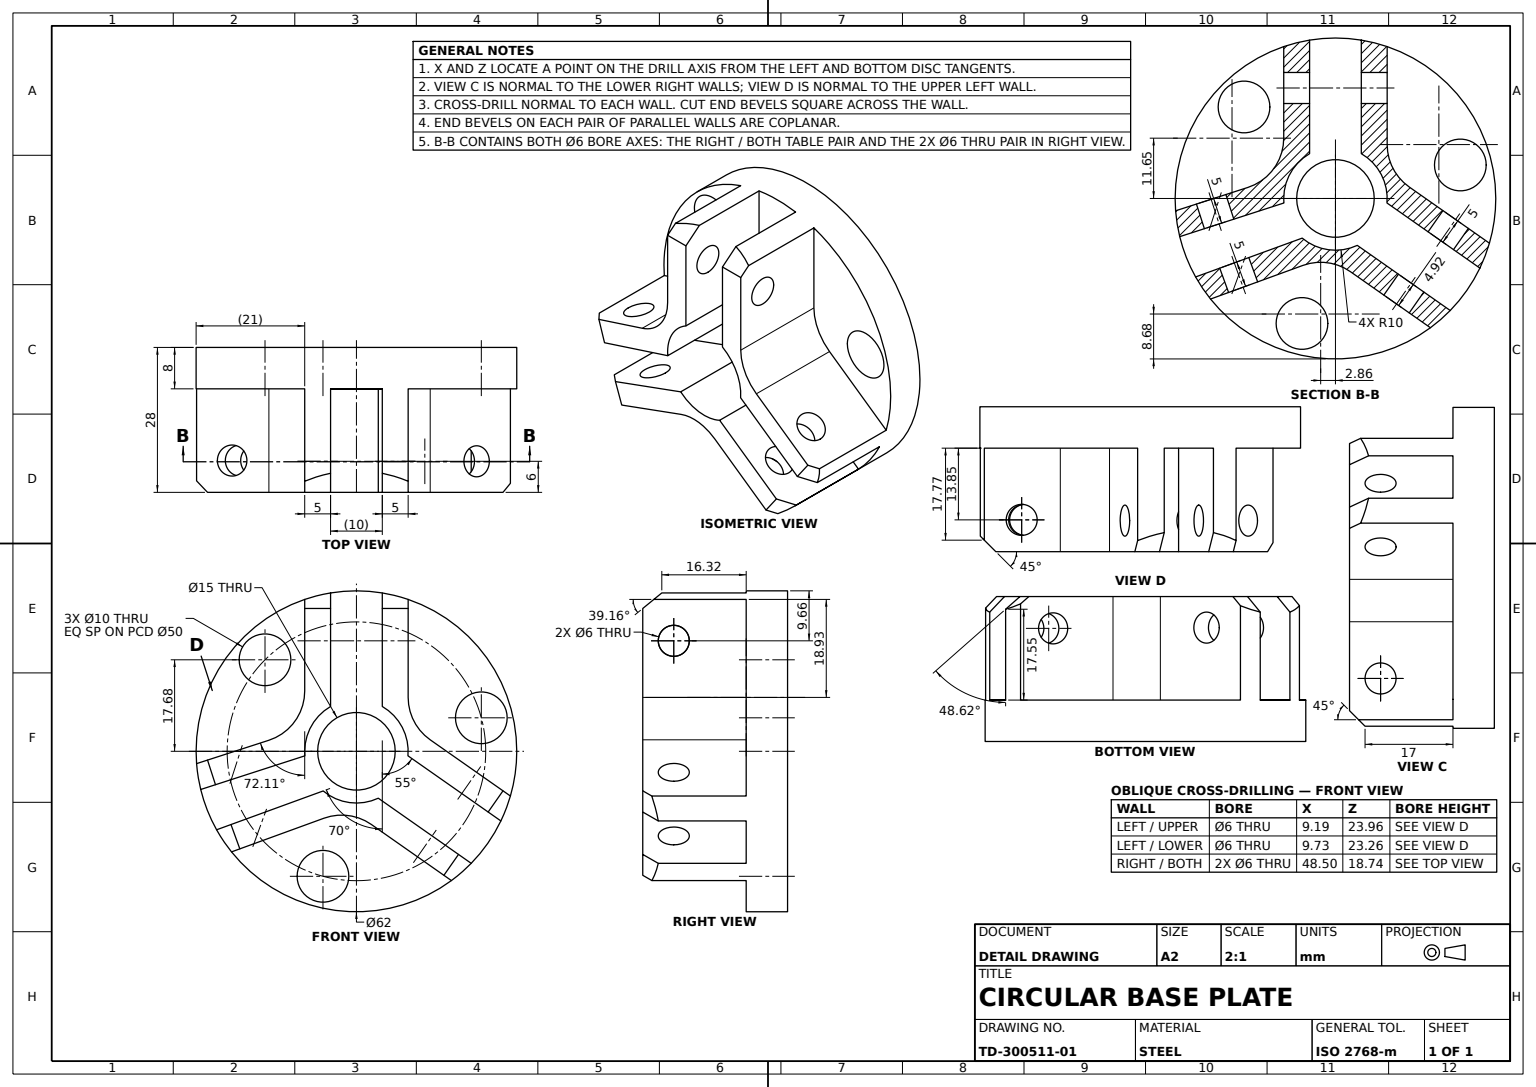
SolidWorks part; units mm, degrees
material "Plain Carbon Steel"
ref_plane "Front Plane" through (0, 0, 0) normal (0, 0, 1) x (1, 0, 0)
ref_plane "Top Plane" through (0, 0, 0) normal (0, 1, 0) x (1, 0, 0)
ref_plane "Right Plane" through (0, 0, 0) normal (1, 0, 0) x (0, 0, -1)
sketch "Base Disc Sketch" plane through (0, 0, 0) normal (0, 0, 1) x (1, 0, 0)
  circle A0 centre (0, 0) radius 31
  dimension "D1" = 62
  dimension "D2" = 62
extrude "Base Disc Ø62" add sketch "Base Disc Sketch" along normal blind 8
sketch "Square Cut Sketch" plane through (0, 0, 8) normal (0, 0, 1) x (1, 0, 0)
  circle A1 centre (-17.6777, 17.6777) radius 5
  circle A2 centre (-6.4705, -24.1481) radius 5
  circle A3 centre (24.1481, 6.4705) radius 5
  arc A4 (25, 0) -> (24.9528, 1.5356) centre (0, 0) ccw
  circle A5 centre (0, 0) radius 31 construction
  dimension "D1" = 10
  dimension "D5" = 10
  dimension "D6" = 10
  dimension "D7" = 10
  dimension "D8" = 10
  dimension "D9" = 10
  dimension "D2" = 25
  dimension "D3" = 24.1481
  dimension "D4" = 25
  dimension "D11" = 6.4705
  dimension "D12" = 17.6777
extrude "Square Cut 10x10" cut sketch "Square Cut Sketch" against normal blind 8 contours A1 | A3 | A2
sketch "Jaws Sketch" plane through (0, 0, 8) normal (0, 0, 1) x (1, 0, 0)
  line L0 (-9.9619, -0.8716) -> (-30.1095, -7.3768)
  line L1 (-5, 10) -> (-5, 30.5941)
  line L3 (5, 10) -> (5, 30.5941)
  line L4 (-5, 10) -> (-5, 8.6603)
  line L5 (5, 10) -> (5, 8.6603)
  line L6 (0, -31) -> (0, -31.7018)
  line L9 (-7.6868, -8.1187) -> (-27.039, -15.1623)
  line L11 (-7.6868, -8.1187) -> (-6.4279, -7.6604)
  line L12 (-10, 11.6499) -> (-10, 29.3428)
  line L13 (11.0594, -1.64) -> (27.9291, -13.4523)
  line L15 (5.3236, -9.8315) -> (22.1934, -21.6438)
  line L16 (5.3236, -9.8315) -> (4.2262, -9.0631)
  line L17 (11.0594, -1.64) -> (9.9619, -0.8716)
  line L19 (10, 10.4113) -> (10, 29.3428)
  line L20 (-16.9274, 2.1336) -> (-30.9085, -2.3806)
  line L23 (-6.2761, -12.9261) -> (-24.153, -19.4328)
  line L25 (14.2642, 2.2198) -> (29.772, -8.6388)
  line L27 (2.8798, -14.1315) -> (18.3651, -24.9744)
  arc A0 (-5, 8.6603) -> (-9.8481, 1.7365) centre (0, 0) ccw
  arc A1 (-6.4279, -7.6604) -> (4.2262, -9.0631) centre (0, 0) ccw
  arc A2 (9.9619, -0.8716) -> (5, 8.6603) centre (0, 0) ccw
  circle A4 centre (0, 0) radius 31 construction
  arc A5 (-5, 8.6603) -> (4.2262, -9.0631) centre (0, 0) ccw
  arc A6 (-6.2761, -12.9261) -> (2.8798, -14.1315) centre (-2.8559, -22.323) cw
  arc A7 (14.2642, 2.2198) -> (10, 10.4113) centre (20, 10.4113) cw
  arc A8 (-10, 11.6499) -> (-16.9274, 2.1336) centre (-20, 11.6499) cw
  arc A9 (9.9619, -0.8716) -> (5, 8.6603) centre (0, 0) ccw
  arc A10 (27.9291, -13.4523) -> (29.772, -8.6388) centre (0, 0) ccw
  arc A11 (18.3651, -24.9744) -> (22.1934, -21.6438) centre (0, 0) ccw
  arc A12 (-30.9085, -2.3806) -> (-30.1095, -7.3768) centre (0, 0) ccw
  arc A13 (10, 29.3428) -> (5, 30.5941) centre (0, 0) ccw
  arc A14 (-27.039, -15.1623) -> (-24.153, -19.4328) centre (0, 0) ccw
  arc A15 (-5, 30.5941) -> (-10, 29.3428) centre (0, 0) ccw
  arc A16 (18.3651, -24.9744) -> (29.772, -8.6388) centre (0, 0) ccw
  arc A17 (10, 29.3428) -> (5, 30.5941) centre (0, 0) ccw
  arc A18 (-30.9085, -2.3806) -> (0, -31) centre (0, 0) ccw
  arc A19 (-5, 30.5941) -> (-10, 29.3428) centre (0, 0) ccw
  circle A20 centre (-17.6777, 17.6777) radius 5 construction
  circle M7 centre (0, 0) radius 31
  dimension "D1" = 20
  dimension "D3" = 20
  dimension "D4" = 10
  dimension "D5" = 62
  dimension "D6" = 62
  dimension "D2" = 47.4496
  dimension "D7" = 0.7503
  dimension "D8" = 0.0381
  dimension "D9" = 0.1139
  dimension "D10" = 2.1613
  dimension "D11" = 1.2589
  dimension "D12" = 0.1518
  dimension "D13" = 1.2761
  dimension "D14" = 2.1441
  dimension "D15" = 1.3463
  dimension "D16" = 13.2308
  dimension "D17" = 3.0705
  dimension "D18" = 49.3795
extrude "Jaws" add sketch "Jaws Sketch" along normal blind 20 contours L12 A8 L20 L0 A5 A0 L4 L1 M7 | L23 A6 L27 L15 L16 A1 L11 L9 M7 | L25 A7 L19 L3 L5 A2 L17 L13 M7
sketch "Jaw Notch 1 Sketch" plane through (5, 0, 0) normal (-1, 0, 0) x (0, 0, 1)
  line L0 (28, 30.5941) -> (28, 27.5941)
  line L1 (28, 11.6499) -> (28, 29.3428) construction
  line L2 (28, 27.5941) -> (24.3164, 30.5941)
  line L3 (28, 30.5941) -> (8, 30.5941) construction
  line L4 (24.3164, 30.5941) -> (28, 30.5941)
  line L5 (8, 8.6603) -> (8, 30.5941) construction
  line L6 (28, 8.6603) -> (8, 8.6603) construction
  dimension "D1" = 16.3164
  dimension "D2" = 18.9339
extrude "Jaw Notch 1" cut sketch "Jaw Notch 1 Sketch" against normal blind 10
sketch "Jaw Notch 2 Sketch" plane through (-5, 0, 0) normal (1, 0, 0) x (0, 0, -1)
  line L0 (-28, 30.5941) -> (-24.3164, 30.5941)
  line L1 (-28, 30.5941) -> (-8, 30.5941) construction
  line L2 (-24.3164, 30.5941) -> (-25.8529, 29.3428) construction
  line L3 (-24.3164, 30.5941) -> (-28, 27.5941)
  line L4 (-28, 27.5941) -> (-28, 30.5941)
extrude "Jaw Notch 2" cut sketch "Jaw Notch 2 Sketch" against normal blind 10
sketch "Jaw Notch 3 Sketch" plane through (2.8679, 4.0958, 0) normal (-0.5736, -0.8192, 0) x (0.8192, -0.5736, 0)
  line L0 (30.5941, 28) -> (30.5941, 25)
  line L1 (30.5941, 28) -> (30.5941, 8) construction
  line L2 (30.5941, 25) -> (27.5941, 28)
  line L3 (10.4645, 28) -> (29.3686, 28) construction
  line L4 (27.5941, 28) -> (30.5941, 28)
  line L5 (30.5941, 28) -> (30.5941, 8) construction
  dimension "D1" = 3
extrude "Jaw Notch 3" cut sketch "Jaw Notch 3 Sketch" against normal blind 10
sketch "Jaw Notch 4 Sketch" plane through (-2.8679, -4.0958, 0) normal (0.5736, 0.8192, 0) x (0.8192, -0.5736, 0)
  line L0 (27.5941, -28) -> (30.5941, -28)
  line L1 (30.5941, -28) -> (30.5941, -25)
  line L2 (29.3428, -26.2513) -> (30.5941, -25) construction
  line L3 (30.5941, -28) -> (30.5941, -8) construction
  line L4 (30.5941, -25) -> (27.5941, -28)
extrude "Jaw Notch 4" cut sketch "Jaw Notch 4 Sketch" against normal blind 10
sketch "Jaw Notch 5 Sketch" plane through (-0.6857, 2.1236, 0) normal (0.3073, -0.9516, 0) x (0.9516, 0.3073, 0)
  line L0 (-30.9196, 28) -> (-27.9196, 28)
  line L1 (-9.9442, 28) -> (-28.9555, 28) construction
  line L2 (-27.9196, 28) -> (-30.9196, 25)
  line L3 (-30.9196, 28) -> (-30.9196, 8) construction
  line L4 (-30.9196, 25) -> (-30.9196, 28)
  line L5 (-9.7478, 28) -> (-9.7478, 8) construction
  dimension "D1" = 18.1717
extrude "Jaw Notch 5" cut sketch "Jaw Notch 5 Sketch" against normal blind 10
sketch "Jaw Notch 6 Sketch" plane through (1.7101, -4.6985, 0) normal (-0.342, 0.9397, 0) x (0.9397, 0.342, 0)
  line L0 (-27.635, -28) -> (-30.5941, -25.5503)
  line L1 (-30.5941, -28) -> (-30.5941, -8) construction
  line L2 (-30.5941, -25.5503) -> (-30.5941, -28)
  line L3 (-30.5941, -28) -> (-27.635, -28)
  dimension "D1" = 2.4497
extrude "Jaw Notch 6" cut sketch "Jaw Notch 6 Sketch" against normal blind 10
sketch "Jaw Hole 1 Sketch" plane through (-0.6857, 2.1236, 0) normal (0.3073, -0.9516, 0) x (0.9516, 0.3073, 0)
  line L0 (-30.9196, 25) -> (-30.9196, 8) construction
  circle A0 centre (-22.9196, 21.8539) radius 3
  dimension "D1" = 6
  dimension "D3" = 6
  dimension "D2" = 8
  dimension "D4" = 13.8539
extrude "Jaw Hole 1 Ø6" cut sketch "Jaw Hole 1 Sketch" against normal blind 10
sketch "Jaw Hole 2 Sketch" plane through (1.7101, -4.6985, 0) normal (-0.342, 0.9397, 0) x (0.9397, 0.342, 0)
  line L0 (-8.6603, -28) -> (-8.6603, -8) construction
  circle A0 centre (-22.6384, -21.8539) radius 3
  dimension "D1" = 6
  dimension "D2" = 6
  dimension "D3" = 13.9781
  dimension "D4" = 6.1461
extrude "Jaw Hole 2 Ø6" cut sketch "Jaw Hole 2 Sketch" against normal blind 10
sketch "Jaw Hole 3 Sketch" plane through (5, 0, 0) normal (-1, 0, 0) x (0, 0, 1)
  line L0 (25.8529, 29.3428) -> (8, 29.3428) construction
  line L1 (28, 11.6499) -> (28, 27.5941) construction
  circle A0 centre (22, 21.3428) radius 3
  dimension "D1" = 6
  dimension "D4" = 6
  dimension "D2" = 8
  dimension "D3" = 6
extrude "Jaw Hole 3 Ø6" cut sketch "Jaw Hole 3 Sketch" against normal blind 10
sketch "Jaw Hole 4 Sketch" plane through (-5, 0, 0) normal (1, 0, 0) x (0, 0, -1)
  circle A0 centre (-22, 21.3428) radius 3
  dimension "D1" = 6
  dimension "D2" = 6
extrude "Jaw Hole 4 Ø6" cut sketch "Jaw Hole 4 Sketch" against normal blind 10
sketch "Jaw Hole 5 Sketch" plane through (2.8679, 4.0958, 0) normal (-0.5736, -0.8192, 0) x (0.8192, -0.5736, 0)
  line L0 (29.3686, 26.2255) -> (29.3686, 8) construction
  line L1 (10.4645, 28) -> (27.5941, 28) construction
  circle A0 centre (21.3686, 22) radius 3
  dimension "D1" = 6
  dimension "D4" = 6
  dimension "D2" = 8
  dimension "D3" = 6
extrude "Jaw Hole 5 Ø6" cut sketch "Jaw Hole 5 Sketch" against normal blind 10
sketch "Jaw Hole 6 Sketch" plane through (-2.8679, -4.0958, 0) normal (0.5736, 0.8192, 0) x (0.8192, -0.5736, 0)
  circle A0 centre (21.3686, -22) radius 3
  dimension "D1" = 6
  dimension "D2" = 6
extrude "Jaw Hole 6 Ø6" cut sketch "Jaw Hole 6 Sketch" against normal blind 10
sketch "Hole Ø15 Sketch" plane through (0, 0, 8) normal (0, 0, 1) x (1, 0, 0)
  circle A0 centre (0, 0) radius 7.5
  dimension "D1" = 15
  dimension "D2" = 15
extrude "Hole Ø15" cut sketch "Hole Ø15 Sketch" against normal blind 10
